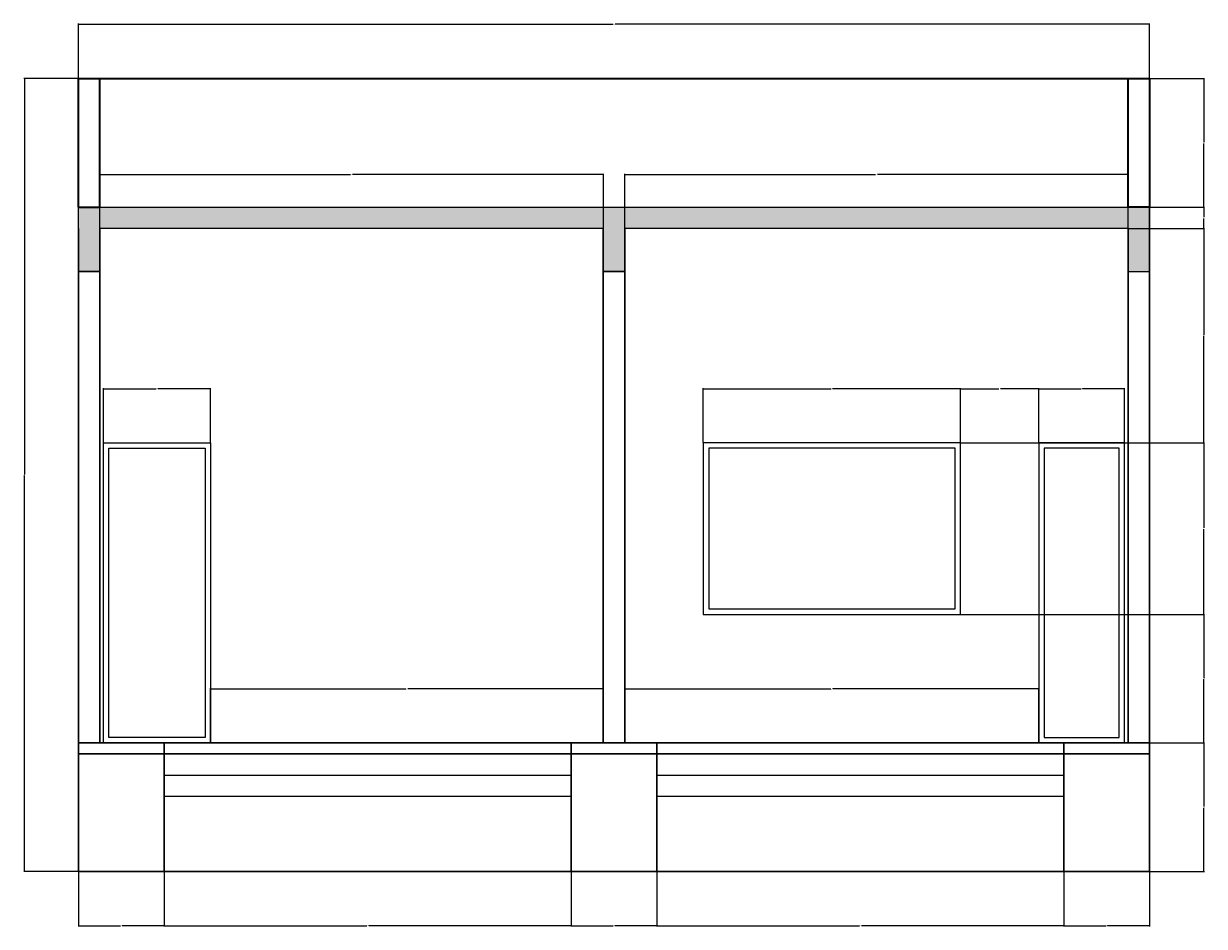
# Model space of a CAD drawing. Units: inches. Extents: x 2156 to 3149, y 1513 to 2286.
# Tile 3 of 5: x 2721 to 3052, y 1551 to 1803. Entities that reach past the tile are written whole.
import ezdxf

# ---------------------------------------------------------------- set-up
doc = ezdxf.new("R2010")
doc.units = ezdxf.units.IN
for name, color, linetype, lineweight in [('A-ANNO-DIMS', 2, 'Continuous', 18), ('A-ELEV', 7, 'Continuous', 30), ('A-ELEV-BASE', 7, 'Continuous', 30), ('A-ELEV-COLS', 7, 'Continuous', 30), ('A-ELEV-DOOR', 3, 'Continuous', 20), ('A-ELEV-GLAZ', 4, 'Continuous', 18), ('A-ELEV-PATT', 18, 'Continuous', 13), ('A-ELEV-STRS', 7, 'Continuous', 20), ('A-ELEV-TRIM', 7, 'Continuous', 20), ('A-ROOF', 7, 'Continuous', 35)]:
    doc.layers.add(name, color=color, linetype=linetype, lineweight=lineweight)
doc.styles.get("Standard").update_dxf_attribs({"font": 'arial.ttf'})
doc.dimstyles.get("Standard").update_dxf_attribs({"dimtxt": 0.18, "dimasz": 0.18, "dimexe": 0.18, "dimexo": 0.0625, "dimgap": 0.09, "dimtad": 0, "dimtih": 1, "dimtoh": 1, "dimdec": 4, "dimzin": 0, "dimdsep": 46, "dimtxsty": 'Standard', "dimcen": 0.09, "dimadec": 0, "dimazin": 0, "dimtfac": 1, "dimtdec": 4, "dimtofl": 0, "dimtmove": 0, "dimatfit": 3, "dimfxl": 1, "dimtolj": 1, "dimtzin": 0, "dimarcsym": 0})

# ---------------------------------------------------------------- blocks, each defined once
blk = doc.blocks.new('*D67')
at = {"layer": 'A-ANNO-DIMS', "color": 0, "lineweight": -2, "transparency": 16777216}
for p, q in [((2736.63, 1787.89), (2736.63, 1803.16)), ((2736.81, 1802.98), (2886.34, 1802.98)), ((3036.45, 1802.98), (2886.92, 1802.98)), ((3036.63, 1787.89), (3036.63, 1803.16))]:
    blk.add_line(p, q, dxfattribs=at)
at = {"layer": 'A-ANNO-DIMS', "color": 0, "transparency": 16777216}
for points in [[(2736.81, 1803.01), (2736.81, 1802.95), (2736.63, 1802.98)], [(3036.45, 1803.01), (3036.45, 1802.95), (3036.63, 1802.98)]]:
    blk.add_solid(points, dxfattribs=at)
at = {"layer": 'Defpoints', "color": 0, "transparency": 16777216}
for p in [(3036.63, 1802.98), (2736.63, 1787.83), (3036.63, 1787.83)]:
    blk.add_point(p, dxfattribs=at)
at = {"layer": 'A-ANNO-DIMS', "color": 0, "transparency": 16777216, "insert": (2886.63, 1802.98), "char_height": 0.18, "attachment_point": 5}
blk.add_mtext('\\A1;300', dxfattribs=at)
blk = doc.blocks.new('*D68')
at = {"layer": 'A-ANNO-DIMS', "color": 0, "lineweight": -2, "transparency": 16777216}
for p, q in [((2736.57, 1787.83), (2721.3, 1787.83)), ((2721.48, 1787.65), (2721.48, 1677.01)), ((2721.48, 1566.01), (2721.48, 1676.65)), ((2736.57, 1565.83), (2721.3, 1565.83))]:
    blk.add_line(p, q, dxfattribs=at)
at = {"layer": 'A-ANNO-DIMS', "color": 0, "transparency": 16777216}
for points in [[(2721.45, 1787.65), (2721.51, 1787.65), (2721.48, 1787.83)], [(2721.45, 1566.01), (2721.51, 1566.01), (2721.48, 1565.83)]]:
    blk.add_solid(points, dxfattribs=at)
at = {"layer": 'Defpoints', "color": 0, "transparency": 16777216}
for p in [(2721.48, 1787.83), (2736.63, 1787.83), (2736.63, 1565.83)]:
    blk.add_point(p, dxfattribs=at)
at = {"layer": 'A-ANNO-DIMS', "color": 0, "transparency": 16777216, "insert": (2721.48, 1676.83), "char_height": 0.18, "attachment_point": 5}
blk.add_mtext('\\A1;222', dxfattribs=at)
blk = doc.blocks.new('*D69')
at = {"layer": 'A-ANNO-DIMS', "color": 0, "lineweight": -2, "transparency": 16777216}
for p, q in [((3036.69, 1601.83), (3051.96, 1601.83)), ((3051.78, 1601.65), (3051.78, 1584.01)), ((3051.78, 1566.01), (3051.78, 1583.65)), ((3036.69, 1565.83), (3051.96, 1565.83))]:
    blk.add_line(p, q, dxfattribs=at)
at = {"layer": 'A-ANNO-DIMS', "color": 0, "transparency": 16777216}
for points in [[(3051.75, 1601.65), (3051.81, 1601.65), (3051.78, 1601.83)], [(3051.75, 1566.01), (3051.81, 1566.01), (3051.78, 1565.83)]]:
    blk.add_solid(points, dxfattribs=at)
at = {"layer": 'Defpoints', "color": 0, "transparency": 16777216}
for p in [(3036.63, 1601.83), (3051.78, 1601.83), (3036.63, 1565.83)]:
    blk.add_point(p, dxfattribs=at)
at = {"layer": 'A-ANNO-DIMS', "color": 0, "transparency": 16777216, "insert": (3051.78, 1583.83), "char_height": 0.18, "attachment_point": 5}
blk.add_mtext('\\A1;36', dxfattribs=at)
blk = doc.blocks.new('*D70')
at = {"layer": 'A-ANNO-DIMS', "color": 0, "lineweight": -2, "transparency": 16777216}
for p, q in [((2983.69, 1637.83), (3051.96, 1637.83)), ((3051.78, 1637.65), (3051.78, 1620.01)), ((3051.78, 1602.01), (3051.78, 1619.65)), ((3036.69, 1601.83), (3051.96, 1601.83))]:
    blk.add_line(p, q, dxfattribs=at)
at = {"layer": 'A-ANNO-DIMS', "color": 0, "transparency": 16777216}
for points in [[(3051.75, 1637.65), (3051.81, 1637.65), (3051.78, 1637.83)], [(3051.75, 1602.01), (3051.81, 1602.01), (3051.78, 1601.83)]]:
    blk.add_solid(points, dxfattribs=at)
at = {"layer": 'Defpoints', "color": 0, "transparency": 16777216}
for p in [(2983.63, 1637.83), (3051.78, 1637.83), (3036.63, 1601.83)]:
    blk.add_point(p, dxfattribs=at)
at = {"layer": 'A-ANNO-DIMS', "color": 0, "transparency": 16777216, "insert": (3051.78, 1619.83), "char_height": 0.18, "attachment_point": 5}
blk.add_mtext('\\A1;36', dxfattribs=at)
blk = doc.blocks.new('*D71')
at = {"layer": 'A-ANNO-DIMS', "color": 0, "lineweight": -2, "transparency": 16777216}
for p, q in [((2983.69, 1685.83), (3051.96, 1685.83)), ((3051.78, 1685.65), (3051.78, 1662.01)), ((3051.78, 1638.01), (3051.78, 1661.65)), ((2983.69, 1637.83), (3051.96, 1637.83))]:
    blk.add_line(p, q, dxfattribs=at)
at = {"layer": 'A-ANNO-DIMS', "color": 0, "transparency": 16777216}
for points in [[(3051.75, 1685.65), (3051.81, 1685.65), (3051.78, 1685.83)], [(3051.75, 1638.01), (3051.81, 1638.01), (3051.78, 1637.83)]]:
    blk.add_solid(points, dxfattribs=at)
at = {"layer": 'Defpoints', "color": 0, "transparency": 16777216}
for p in [(2983.63, 1685.83), (3051.78, 1685.83), (2983.63, 1637.83)]:
    blk.add_point(p, dxfattribs=at)
at = {"layer": 'A-ANNO-DIMS', "color": 0, "transparency": 16777216, "insert": (3051.78, 1661.83), "char_height": 0.18, "attachment_point": 5}
blk.add_mtext('\\A1;48', dxfattribs=at)
blk = doc.blocks.new('*D72')
at = {"layer": 'A-ANNO-DIMS', "color": 0, "lineweight": -2, "transparency": 16777216}
for p, q in [((3030.69, 1745.83), (3051.96, 1745.83)), ((3051.78, 1745.65), (3051.78, 1716.01)), ((3051.78, 1686.01), (3051.78, 1715.65)), ((2983.69, 1685.83), (3051.96, 1685.83))]:
    blk.add_line(p, q, dxfattribs=at)
at = {"layer": 'A-ANNO-DIMS', "color": 0, "transparency": 16777216}
for points in [[(3051.75, 1745.65), (3051.81, 1745.65), (3051.78, 1745.83)], [(3051.75, 1686.01), (3051.81, 1686.01), (3051.78, 1685.83)]]:
    blk.add_solid(points, dxfattribs=at)
at = {"layer": 'Defpoints', "color": 0, "transparency": 16777216}
for p in [(3030.63, 1745.83), (3051.78, 1745.83), (2983.63, 1685.83)]:
    blk.add_point(p, dxfattribs=at)
at = {"layer": 'A-ANNO-DIMS', "color": 0, "transparency": 16777216, "insert": (3051.78, 1715.83), "char_height": 0.18, "attachment_point": 5}
blk.add_mtext('\\A1;60', dxfattribs=at)
blk = doc.blocks.new('*D73')
at = {"layer": 'A-ANNO-DIMS', "color": 0, "lineweight": -2, "transparency": 16777216}
for p, q in [((3036.69, 1751.83), (3051.96, 1751.83)), ((3051.78, 1751.65), (3051.78, 1749.01)), ((3051.78, 1746.01), (3051.78, 1748.65)), ((3030.69, 1745.83), (3051.96, 1745.83))]:
    blk.add_line(p, q, dxfattribs=at)
at = {"layer": 'A-ANNO-DIMS', "color": 0, "transparency": 16777216}
for points in [[(3051.75, 1751.65), (3051.81, 1751.65), (3051.78, 1751.83)], [(3051.75, 1746.01), (3051.81, 1746.01), (3051.78, 1745.83)]]:
    blk.add_solid(points, dxfattribs=at)
at = {"layer": 'Defpoints', "color": 0, "transparency": 16777216}
for p in [(3036.63, 1751.83), (3051.78, 1751.83), (3030.63, 1745.83)]:
    blk.add_point(p, dxfattribs=at)
at = {"layer": 'A-ANNO-DIMS', "color": 0, "transparency": 16777216, "insert": (3051.78, 1748.83), "char_height": 0.18, "attachment_point": 5}
blk.add_mtext('\\A1;6', dxfattribs=at)
blk = doc.blocks.new('*D74')
at = {"layer": 'A-ANNO-DIMS', "color": 0, "lineweight": -2, "transparency": 16777216}
for p, q in [((3036.69, 1787.83), (3051.96, 1787.83)), ((3051.78, 1787.65), (3051.78, 1770.01)), ((3051.78, 1752.01), (3051.78, 1769.65)), ((3036.69, 1751.83), (3051.96, 1751.83))]:
    blk.add_line(p, q, dxfattribs=at)
at = {"layer": 'A-ANNO-DIMS', "color": 0, "transparency": 16777216}
for points in [[(3051.75, 1787.65), (3051.81, 1787.65), (3051.78, 1787.83)], [(3051.75, 1752.01), (3051.81, 1752.01), (3051.78, 1751.83)]]:
    blk.add_solid(points, dxfattribs=at)
at = {"layer": 'Defpoints', "color": 0, "transparency": 16777216}
for p in [(3036.63, 1787.83), (3051.78, 1787.83), (3036.63, 1751.83)]:
    blk.add_point(p, dxfattribs=at)
at = {"layer": 'A-ANNO-DIMS', "color": 0, "transparency": 16777216, "insert": (3051.78, 1769.83), "char_height": 0.18, "attachment_point": 5}
blk.add_mtext('\\A1;36', dxfattribs=at)
blk = doc.blocks.new('*D75')
at = {"layer": 'A-ANNO-DIMS', "color": 0, "lineweight": -2, "transparency": 16777216}
for p, q in [((2743.63, 1685.89), (2743.63, 1701.16)), ((2743.81, 1700.98), (2758.41, 1700.98)), ((2773.45, 1700.98), (2758.85, 1700.98)), ((2773.63, 1685.89), (2773.63, 1701.16))]:
    blk.add_line(p, q, dxfattribs=at)
at = {"layer": 'A-ANNO-DIMS', "color": 0, "transparency": 16777216}
for points in [[(2743.81, 1701.01), (2743.81, 1700.95), (2743.63, 1700.98)], [(2773.45, 1701.01), (2773.45, 1700.95), (2773.63, 1700.98)]]:
    blk.add_solid(points, dxfattribs=at)
at = {"layer": 'Defpoints', "color": 0, "transparency": 16777216}
for p in [(2773.63, 1700.98), (2743.63, 1685.83), (2773.63, 1685.83)]:
    blk.add_point(p, dxfattribs=at)
at = {"layer": 'A-ANNO-DIMS', "color": 0, "transparency": 16777216, "insert": (2758.63, 1700.98), "char_height": 0.18, "attachment_point": 5}
blk.add_mtext('\\A1;30', dxfattribs=at)
blk = doc.blocks.new('*D76')
at = {"layer": 'A-ANNO-DIMS', "color": 0, "lineweight": -2, "transparency": 16777216}
for p, q in [((2911.63, 1685.89), (2911.63, 1701.16)), ((2911.81, 1700.98), (2947.41, 1700.98)), ((2983.45, 1700.98), (2947.85, 1700.98)), ((2983.63, 1685.89), (2983.63, 1701.16))]:
    blk.add_line(p, q, dxfattribs=at)
at = {"layer": 'A-ANNO-DIMS', "color": 0, "transparency": 16777216}
for points in [[(2911.81, 1701.01), (2911.81, 1700.95), (2911.63, 1700.98)], [(2983.45, 1701.01), (2983.45, 1700.95), (2983.63, 1700.98)]]:
    blk.add_solid(points, dxfattribs=at)
at = {"layer": 'Defpoints', "color": 0, "transparency": 16777216}
for p in [(2983.63, 1700.98), (2911.63, 1685.83), (2983.63, 1685.83)]:
    blk.add_point(p, dxfattribs=at)
at = {"layer": 'A-ANNO-DIMS', "color": 0, "transparency": 16777216, "insert": (2947.63, 1700.98), "char_height": 0.18, "attachment_point": 5}
blk.add_mtext('\\A1;72', dxfattribs=at)
blk = doc.blocks.new('*D77')
at = {"layer": 'A-ANNO-DIMS', "color": 0, "lineweight": -2, "transparency": 16777216}
for p, q in [((2983.63, 1685.89), (2983.63, 1701.16)), ((2983.81, 1700.98), (2994.41, 1700.98)), ((3005.45, 1700.98), (2994.85, 1700.98)), ((3005.63, 1685.89), (3005.63, 1701.16))]:
    blk.add_line(p, q, dxfattribs=at)
at = {"layer": 'A-ANNO-DIMS', "color": 0, "transparency": 16777216}
for points in [[(2983.81, 1701.01), (2983.81, 1700.95), (2983.63, 1700.98)], [(3005.45, 1701.01), (3005.45, 1700.95), (3005.63, 1700.98)]]:
    blk.add_solid(points, dxfattribs=at)
at = {"layer": 'Defpoints', "color": 0, "transparency": 16777216}
for p in [(3005.63, 1700.98), (2983.63, 1685.83), (3005.63, 1685.83)]:
    blk.add_point(p, dxfattribs=at)
at = {"layer": 'A-ANNO-DIMS', "color": 0, "transparency": 16777216, "insert": (2994.63, 1700.98), "char_height": 0.18, "attachment_point": 5}
blk.add_mtext('\\A1;22', dxfattribs=at)
blk = doc.blocks.new('*D78')
at = {"layer": 'A-ANNO-DIMS', "color": 0, "lineweight": -2, "transparency": 16777216}
for p, q in [((3005.63, 1685.89), (3005.63, 1701.16)), ((3005.81, 1700.98), (3017.41, 1700.98)), ((3029.45, 1700.98), (3017.85, 1700.98)), ((3029.63, 1685.89), (3029.63, 1701.16))]:
    blk.add_line(p, q, dxfattribs=at)
at = {"layer": 'A-ANNO-DIMS', "color": 0, "transparency": 16777216}
for points in [[(3005.81, 1701.01), (3005.81, 1700.95), (3005.63, 1700.98)], [(3029.45, 1701.01), (3029.45, 1700.95), (3029.63, 1700.98)]]:
    blk.add_solid(points, dxfattribs=at)
at = {"layer": 'Defpoints', "color": 0, "transparency": 16777216}
for p in [(3029.63, 1700.98), (3005.63, 1685.83), (3029.63, 1685.83)]:
    blk.add_point(p, dxfattribs=at)
at = {"layer": 'A-ANNO-DIMS', "color": 0, "transparency": 16777216, "insert": (3017.63, 1700.98), "char_height": 0.18, "attachment_point": 5}
blk.add_mtext('\\A1;24', dxfattribs=at)
blk = doc.blocks.new('*D79')
at = {"layer": 'A-ANNO-DIMS', "color": 0, "lineweight": -2, "transparency": 16777216}
for p, q in [((2773.63, 1601.89), (2773.63, 1617.16)), ((2883.63, 1601.89), (2883.63, 1617.16)), ((2773.81, 1616.98), (2828.35, 1616.98)), ((2883.45, 1616.98), (2828.91, 1616.98))]:
    blk.add_line(p, q, dxfattribs=at)
at = {"layer": 'A-ANNO-DIMS', "color": 0, "transparency": 16777216}
for points in [[(2773.81, 1617.01), (2773.81, 1616.95), (2773.63, 1616.98)], [(2883.45, 1617.01), (2883.45, 1616.95), (2883.63, 1616.98)]]:
    blk.add_solid(points, dxfattribs=at)
at = {"layer": 'Defpoints', "color": 0, "transparency": 16777216}
for p in [(2883.63, 1616.98), (2773.63, 1601.83), (2883.63, 1601.83)]:
    blk.add_point(p, dxfattribs=at)
at = {"layer": 'A-ANNO-DIMS', "color": 0, "transparency": 16777216, "insert": (2828.63, 1616.98), "char_height": 0.18, "attachment_point": 5}
blk.add_mtext('\\A1;110', dxfattribs=at)
blk = doc.blocks.new('*D80')
at = {"layer": 'A-ANNO-DIMS', "color": 0, "lineweight": -2, "transparency": 16777216}
for p, q in [((2889.63, 1601.89), (2889.63, 1617.16)), ((3005.63, 1601.89), (3005.63, 1617.16)), ((2889.81, 1616.98), (2947.35, 1616.98)), ((3005.45, 1616.98), (2947.91, 1616.98))]:
    blk.add_line(p, q, dxfattribs=at)
at = {"layer": 'A-ANNO-DIMS', "color": 0, "transparency": 16777216}
for points in [[(2889.81, 1617.01), (2889.81, 1616.95), (2889.63, 1616.98)], [(3005.45, 1617.01), (3005.45, 1616.95), (3005.63, 1616.98)]]:
    blk.add_solid(points, dxfattribs=at)
at = {"layer": 'Defpoints', "color": 0, "transparency": 16777216}
for p in [(3005.63, 1616.98), (2889.63, 1601.83), (3005.63, 1601.83)]:
    blk.add_point(p, dxfattribs=at)
at = {"layer": 'A-ANNO-DIMS', "color": 0, "transparency": 16777216, "insert": (2947.63, 1616.98), "char_height": 0.18, "attachment_point": 5}
blk.add_mtext('\\A1;116', dxfattribs=at)
blk = doc.blocks.new('*D81')
at = {"layer": 'A-ANNO-DIMS', "color": 0, "lineweight": -2, "transparency": 16777216}
for p, q in [((2742.63, 1745.89), (2742.63, 1761.16)), ((2742.81, 1760.98), (2812.86, 1760.98)), ((2883.45, 1760.98), (2813.39, 1760.98)), ((2883.63, 1745.89), (2883.63, 1761.16))]:
    blk.add_line(p, q, dxfattribs=at)
at = {"layer": 'A-ANNO-DIMS', "color": 0, "transparency": 16777216}
for points in [[(2742.81, 1761.01), (2742.81, 1760.95), (2742.63, 1760.98)], [(2883.45, 1761.01), (2883.45, 1760.95), (2883.63, 1760.98)]]:
    blk.add_solid(points, dxfattribs=at)
at = {"layer": 'Defpoints', "color": 0, "transparency": 16777216}
for p in [(2883.63, 1760.98), (2742.63, 1745.83), (2883.63, 1745.83)]:
    blk.add_point(p, dxfattribs=at)
at = {"layer": 'A-ANNO-DIMS', "color": 0, "transparency": 16777216, "insert": (2813.13, 1760.98), "char_height": 0.18, "attachment_point": 5}
blk.add_mtext('\\A1;141', dxfattribs=at)
blk = doc.blocks.new('*D82')
at = {"layer": 'A-ANNO-DIMS', "color": 0, "lineweight": -2, "transparency": 16777216}
for p, q in [((2889.63, 1745.89), (2889.63, 1761.16)), ((2889.81, 1760.98), (2959.86, 1760.98)), ((3030.45, 1760.98), (2960.39, 1760.98)), ((3030.63, 1745.89), (3030.63, 1761.16))]:
    blk.add_line(p, q, dxfattribs=at)
at = {"layer": 'A-ANNO-DIMS', "color": 0, "transparency": 16777216}
for points in [[(2889.81, 1761.01), (2889.81, 1760.95), (2889.63, 1760.98)], [(3030.45, 1761.01), (3030.45, 1760.95), (3030.63, 1760.98)]]:
    blk.add_solid(points, dxfattribs=at)
at = {"layer": 'Defpoints', "color": 0, "transparency": 16777216}
for p in [(3030.63, 1760.98), (2889.63, 1745.83), (3030.63, 1745.83)]:
    blk.add_point(p, dxfattribs=at)
at = {"layer": 'A-ANNO-DIMS', "color": 0, "transparency": 16777216, "insert": (2960.13, 1760.98), "char_height": 0.18, "attachment_point": 5}
blk.add_mtext('\\A1;141', dxfattribs=at)
blk = doc.blocks.new('*D83')
at = {"layer": 'A-ANNO-DIMS', "color": 0, "lineweight": -2, "transparency": 16777216}
for p, q in [((2736.63, 1565.77), (2736.63, 1550.5)), ((2760.63, 1565.77), (2760.63, 1550.5)), ((2736.81, 1550.68), (2748.41, 1550.68)), ((2760.45, 1550.68), (2748.85, 1550.68))]:
    blk.add_line(p, q, dxfattribs=at)
at = {"layer": 'A-ANNO-DIMS', "color": 0, "transparency": 16777216}
for points in [[(2736.81, 1550.71), (2736.81, 1550.65), (2736.63, 1550.68)], [(2760.45, 1550.71), (2760.45, 1550.65), (2760.63, 1550.68)]]:
    blk.add_solid(points, dxfattribs=at)
at = {"layer": 'Defpoints', "color": 0, "transparency": 16777216}
for p in [(2736.63, 1565.83), (2760.63, 1565.83), (2760.63, 1550.68)]:
    blk.add_point(p, dxfattribs=at)
at = {"layer": 'A-ANNO-DIMS', "color": 0, "transparency": 16777216, "insert": (2748.63, 1550.68), "char_height": 0.18, "attachment_point": 5}
blk.add_mtext('\\A1;24', dxfattribs=at)
blk = doc.blocks.new('*D84')
at = {"layer": 'A-ANNO-DIMS', "color": 0, "lineweight": -2, "transparency": 16777216}
for p, q in [((2760.63, 1565.77), (2760.63, 1550.5)), ((2874.63, 1565.77), (2874.63, 1550.5)), ((2760.81, 1550.68), (2817.35, 1550.68)), ((2874.45, 1550.68), (2817.91, 1550.68))]:
    blk.add_line(p, q, dxfattribs=at)
at = {"layer": 'A-ANNO-DIMS', "color": 0, "transparency": 16777216}
for points in [[(2760.81, 1550.71), (2760.81, 1550.65), (2760.63, 1550.68)], [(2874.45, 1550.71), (2874.45, 1550.65), (2874.63, 1550.68)]]:
    blk.add_solid(points, dxfattribs=at)
at = {"layer": 'Defpoints', "color": 0, "transparency": 16777216}
for p in [(2760.63, 1565.83), (2874.63, 1565.83), (2874.63, 1550.68)]:
    blk.add_point(p, dxfattribs=at)
at = {"layer": 'A-ANNO-DIMS', "color": 0, "transparency": 16777216, "insert": (2817.63, 1550.68), "char_height": 0.18, "attachment_point": 5}
blk.add_mtext('\\A1;114', dxfattribs=at)
blk = doc.blocks.new('*D85')
at = {"layer": 'A-ANNO-DIMS', "color": 0, "lineweight": -2, "transparency": 16777216}
for p, q in [((2874.63, 1565.77), (2874.63, 1550.5)), ((2898.63, 1565.77), (2898.63, 1550.5)), ((2874.81, 1550.68), (2886.41, 1550.68)), ((2898.45, 1550.68), (2886.85, 1550.68))]:
    blk.add_line(p, q, dxfattribs=at)
at = {"layer": 'A-ANNO-DIMS', "color": 0, "transparency": 16777216}
for points in [[(2874.81, 1550.71), (2874.81, 1550.65), (2874.63, 1550.68)], [(2898.45, 1550.71), (2898.45, 1550.65), (2898.63, 1550.68)]]:
    blk.add_solid(points, dxfattribs=at)
at = {"layer": 'Defpoints', "color": 0, "transparency": 16777216}
for p in [(2874.63, 1565.83), (2898.63, 1565.83), (2898.63, 1550.68)]:
    blk.add_point(p, dxfattribs=at)
at = {"layer": 'A-ANNO-DIMS', "color": 0, "transparency": 16777216, "insert": (2886.63, 1550.68), "char_height": 0.18, "attachment_point": 5}
blk.add_mtext('\\A1;24', dxfattribs=at)
blk = doc.blocks.new('*D86')
at = {"layer": 'A-ANNO-DIMS', "color": 0, "lineweight": -2, "transparency": 16777216}
for p, q in [((2898.63, 1565.77), (2898.63, 1550.5)), ((3012.63, 1565.77), (3012.63, 1550.5)), ((2898.81, 1550.68), (2955.35, 1550.68)), ((3012.45, 1550.68), (2955.91, 1550.68))]:
    blk.add_line(p, q, dxfattribs=at)
at = {"layer": 'A-ANNO-DIMS', "color": 0, "transparency": 16777216}
for points in [[(2898.81, 1550.71), (2898.81, 1550.65), (2898.63, 1550.68)], [(3012.45, 1550.71), (3012.45, 1550.65), (3012.63, 1550.68)]]:
    blk.add_solid(points, dxfattribs=at)
at = {"layer": 'Defpoints', "color": 0, "transparency": 16777216}
for p in [(2898.63, 1565.83), (3012.63, 1565.83), (3012.63, 1550.68)]:
    blk.add_point(p, dxfattribs=at)
at = {"layer": 'A-ANNO-DIMS', "color": 0, "transparency": 16777216, "insert": (2955.63, 1550.68), "char_height": 0.18, "attachment_point": 5}
blk.add_mtext('\\A1;114', dxfattribs=at)
blk = doc.blocks.new('*D87')
at = {"layer": 'A-ANNO-DIMS', "color": 0, "lineweight": -2, "transparency": 16777216}
for p, q in [((3012.63, 1565.77), (3012.63, 1550.5)), ((3036.63, 1565.77), (3036.63, 1550.5)), ((3012.81, 1550.68), (3024.41, 1550.68)), ((3036.45, 1550.68), (3024.85, 1550.68))]:
    blk.add_line(p, q, dxfattribs=at)
at = {"layer": 'A-ANNO-DIMS', "color": 0, "transparency": 16777216}
for points in [[(3012.81, 1550.71), (3012.81, 1550.65), (3012.63, 1550.68)], [(3036.45, 1550.71), (3036.45, 1550.65), (3036.63, 1550.68)]]:
    blk.add_solid(points, dxfattribs=at)
at = {"layer": 'Defpoints', "color": 0, "transparency": 16777216}
for p in [(3012.63, 1565.83), (3036.63, 1565.83), (3036.63, 1550.68)]:
    blk.add_point(p, dxfattribs=at)
at = {"layer": 'A-ANNO-DIMS', "color": 0, "transparency": 16777216, "insert": (3024.63, 1550.68), "char_height": 0.18, "attachment_point": 5}
blk.add_mtext('\\A1;24', dxfattribs=at)

msp = doc.modelspace()

# ---------------------------------------------------------------- hatches: boundary and pattern name
at = {"layer": 'A-ELEV-PATT'}
h = msp.add_hatch(color=256, dxfattribs=at)
h.dxf.hatch_style = 1
h.paths.add_polyline_path([(2889.628, 1745.832), (3030.628, 1745.832), (3030.628, 1733.832), (3036.628, 1733.832), (3036.628, 1751.832), (3030.628, 1751.832), (2736.628, 1751.832), (2736.628, 1745.832), (2736.628, 1733.832), (2742.628, 1733.832), (2742.628, 1745.832), (2883.628, 1745.832), (2883.628, 1733.832), (2889.628, 1733.832)])

# ---------------------------------------------------------------- linework, layer by layer
at = {"layer": 'A-ELEV'}
for p, q in [((3036.628, 1751.832), (3036.628, 1601.832)), ((2736.628, 1601.832), (2736.628, 1745.832)), ((2742.628, 1601.832), (2743.628, 1601.832)), ((3030.628, 1601.832), (3029.628, 1601.832)), ((3036.628, 1601.832), (3030.628, 1601.832))]:
    msp.add_line(p, q, dxfattribs=at)
at = {"layer": 'A-ELEV-BASE'}
for p, q in [((2736.628, 1565.832), (2736.628, 1601.832)), ((2736.628, 1601.832), (2760.628, 1601.832)), ((2736.628, 1601.832), (2736.628, 1598.832)), ((2760.628, 1601.832), (2760.628, 1565.832)), ((2760.628, 1601.832), (3012.628, 1601.832)), ((2898.628, 1601.832), (2874.628, 1601.832)), ((2874.628, 1601.832), (2874.628, 1598.832)), ((2874.628, 1601.832), (2886.628, 1601.832)), ((2898.628, 1565.832), (2898.628, 1601.832)), ((3036.628, 1601.832), (3012.628, 1601.832)), ((3012.628, 1601.832), (3012.628, 1565.832)), ((3012.628, 1601.832), (3012.628, 1598.832)), ((3036.628, 1565.832), (3036.628, 1601.832)), ((2736.628, 1598.832), (2760.628, 1598.832)), ((3012.628, 1598.832), (2760.628, 1598.832)), ((2760.628, 1598.832), (3036.628, 1598.832)), ((2886.628, 1598.832), (2874.628, 1598.832)), ((2874.628, 1598.832), (2874.628, 1565.832)), ((2760.628, 1565.832), (2736.628, 1565.832)), ((2736.628, 1565.832), (3036.628, 1565.832)), ((2874.628, 1565.832), (2898.628, 1565.832))]:
    msp.add_line(p, q, dxfattribs=at)
at = {"layer": 'A-ELEV-COLS'}
for p, q in [((2742.628, 1745.832), (2742.628, 1601.832)), ((2883.628, 1601.832), (2883.628, 1745.832)), ((2889.628, 1601.832), (2889.628, 1745.832)), ((3030.628, 1601.832), (3030.628, 1745.832)), ((2883.628, 1733.832), (2889.628, 1733.832))]:
    msp.add_line(p, q, dxfattribs=at)
at = {"layer": 'A-ELEV-DOOR'}
for p, q in [((2743.628, 1601.832), (2743.628, 1685.832)), ((2743.628, 1685.832), (2773.628, 1685.832)), ((2745.128, 1603.332), (2745.128, 1684.332)), ((2745.128, 1684.332), (2772.128, 1684.332)), ((2772.128, 1684.332), (2772.128, 1603.332)), ((2773.628, 1685.832), (2773.628, 1601.832)), ((3029.628, 1685.832), (3005.628, 1685.832)), ((3005.628, 1685.832), (3005.628, 1601.832)), ((3007.128, 1684.332), (3007.128, 1603.332)), ((3028.128, 1684.332), (3007.128, 1684.332)), ((3028.128, 1603.332), (3028.128, 1684.332)), ((3029.628, 1601.832), (3029.628, 1685.832)), ((2773.628, 1601.832), (2743.628, 1601.832)), ((2772.128, 1603.332), (2745.128, 1603.332)), ((3007.128, 1603.332), (3028.128, 1603.332)), ((3007.128, 1601.832), (3028.128, 1601.832))]:
    msp.add_line(p, q, dxfattribs=at)
at = {"layer": 'A-ELEV-GLAZ'}
for p, q in [((2983.628, 1685.832), (2911.628, 1685.832)), ((2911.628, 1685.832), (2911.628, 1637.832)), ((2913.128, 1684.332), (2913.128, 1639.332)), ((2982.128, 1684.332), (2913.128, 1684.332)), ((2982.128, 1639.332), (2982.128, 1684.332)), ((2983.628, 1637.832), (2983.628, 1685.832)), ((2911.628, 1637.832), (2983.628, 1637.832)), ((2913.128, 1639.332), (2982.128, 1639.332))]:
    msp.add_line(p, q, dxfattribs=at)
at = {"layer": 'A-ELEV-STRS'}
for p, q in [((2760.628, 1598.832), (2760.628, 1592.832)), ((2760.628, 1592.832), (2874.628, 1592.832)), ((2898.628, 1592.832), (3012.628, 1592.832)), ((3012.628, 1592.832), (3012.628, 1586.832)), ((2874.628, 1586.832), (2760.628, 1586.832)), ((3012.628, 1586.832), (2898.628, 1586.832))]:
    msp.add_line(p, q, dxfattribs=at)
at = {"layer": 'A-ELEV-TRIM'}
for p, q in [((2736.628, 1745.832), (2736.628, 1751.832)), ((2736.628, 1751.832), (3036.628, 1751.832)), ((2883.628, 1745.832), (2742.628, 1745.832)), ((2742.628, 1745.832), (2742.628, 1733.832)), ((3030.628, 1745.832), (2889.628, 1745.832)), ((2742.628, 1733.832), (2736.628, 1733.832)), ((2736.628, 1733.832), (2742.628, 1733.832)), ((3030.628, 1733.832), (3036.628, 1733.832))]:
    msp.add_line(p, q, dxfattribs=at)
at = {"layer": 'A-ROOF'}
for p, q in [((2736.628, 1751.832), (2736.628, 1787.832)), ((2736.628, 1787.832), (3036.628, 1787.832)), ((2742.628, 1751.832), (2742.628, 1787.832)), ((3030.628, 1751.832), (3030.628, 1787.832)), ((3036.628, 1787.832), (3036.628, 1751.832)), ((2736.628, 1751.832), (2742.628, 1751.832)), ((3036.628, 1751.832), (3030.628, 1751.832))]:
    msp.add_line(p, q, dxfattribs=at)

# ---------------------------------------------------------------- dimensions: what is measured, and where the dimension line sits
at = {"layer": 'A-ANNO-DIMS'}
for base, p1, p2, picture, middle in [((3036.628, 1802.982), (2736.628, 1787.832), (3036.628, 1787.832), '*D67', (2886.628, 1802.982)), ((2883.628, 1760.982), (2742.628, 1745.832), (2883.628, 1745.832), '*D81', (2813.128, 1760.982)), ((3030.628, 1760.982), (2889.628, 1745.832), (3030.628, 1745.832), '*D82', (2960.128, 1760.982)), ((2773.628, 1700.982), (2743.628, 1685.832), (2773.628, 1685.832), '*D75', (2758.628, 1700.982)), ((3005.628, 1700.982), (2983.628, 1685.832), (3005.628, 1685.832), '*D77', (2994.628, 1700.982)), ((3029.628, 1700.982), (3005.628, 1685.832), (3029.628, 1685.832), '*D78', (3017.628, 1700.982)), ((2883.628, 1616.982), (2773.628, 1601.832), (2883.628, 1601.832), '*D79', (2828.628, 1616.982)), ((3005.628, 1616.982), (2889.628, 1601.832), (3005.628, 1601.832), '*D80', (2947.628, 1616.982)), ((2760.628, 1550.682), (2736.628, 1565.832), (2760.628, 1565.832), '*D83', (2748.628, 1550.682)), ((2874.628, 1550.682), (2760.628, 1565.832), (2874.628, 1565.832), '*D84', (2817.628, 1550.682)), ((2898.628, 1550.682), (2874.628, 1565.832), (2898.628, 1565.832), '*D85', (2886.628, 1550.682)), ((3012.628, 1550.682), (2898.628, 1565.832), (3012.628, 1565.832), '*D86', (2955.628, 1550.682)), ((3036.628, 1550.682), (3012.628, 1565.832), (3036.628, 1565.832), '*D87', (3024.628, 1550.682))]:
    dim = msp.add_linear_dim(base=base, p1=p1, p2=p2, dimstyle='Standard', override={"dimdec": 0, "dimlfac": 1, "dimrnd": 0, "dimzin": 0, "dimdsep": 46, "dimlunit": 2}, dxfattribs=at)
    dim.commit()
    dim.dimension.update_dxf_attribs({"geometry": picture, "text_midpoint": middle})
for base, p1, p2, angle, picture, middle in [((2721.478, 1787.832), (2736.628, 1565.832), (2736.628, 1787.832), 90, '*D68', (2721.478, 1676.832)), ((3051.778, 1787.832), (3036.628, 1751.832), (3036.628, 1787.832), 90, '*D74', (3051.778, 1769.832)), ((3051.778, 1751.832), (3030.628, 1745.832), (3036.628, 1751.832), 90, '*D73', (3051.778, 1748.832)), ((3051.778, 1745.832), (2983.628, 1685.832), (3030.628, 1745.832), 90, '*D72', (3051.778, 1715.832)), ((2983.628, 1700.982), (2911.628, 1685.832), (2983.628, 1685.832), 0, '*D76', (2947.628, 1700.982)), ((3051.778, 1685.832), (2983.628, 1637.832), (2983.628, 1685.832), 90, '*D71', (3051.778, 1661.832)), ((3051.778, 1637.832), (3036.628, 1601.832), (2983.628, 1637.832), 90, '*D70', (3051.778, 1619.832)), ((3051.778, 1601.832), (3036.628, 1565.832), (3036.628, 1601.832), 90, '*D69', (3051.778, 1583.832))]:
    dim = msp.add_linear_dim(base=base, p1=p1, p2=p2, angle=angle, dimstyle='Standard', override={"dimdec": 0, "dimlfac": 1, "dimrnd": 0, "dimzin": 0, "dimdsep": 46, "dimlunit": 2}, dxfattribs=at)
    dim.commit()
    dim.dimension.update_dxf_attribs({"geometry": picture, "text_midpoint": middle})

doc.saveas('drawing.dxf')
